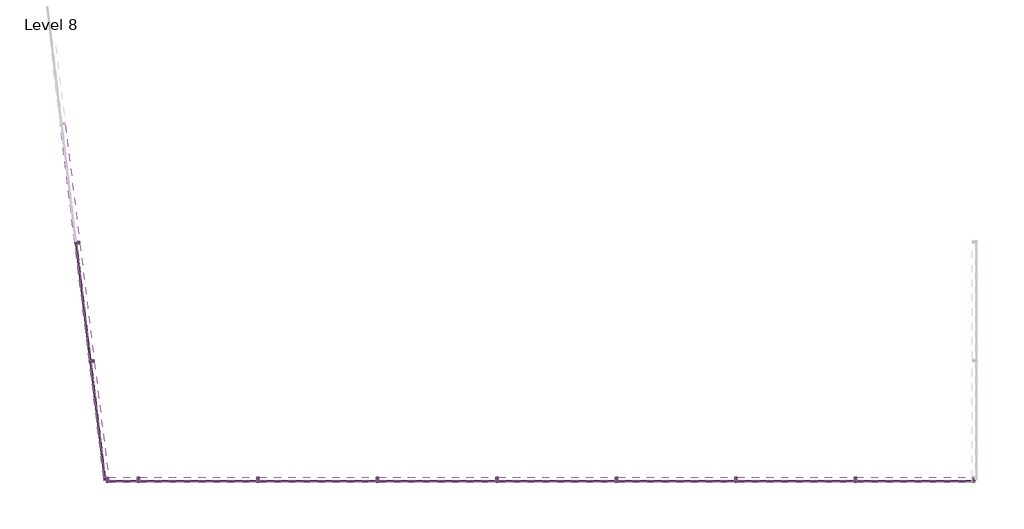
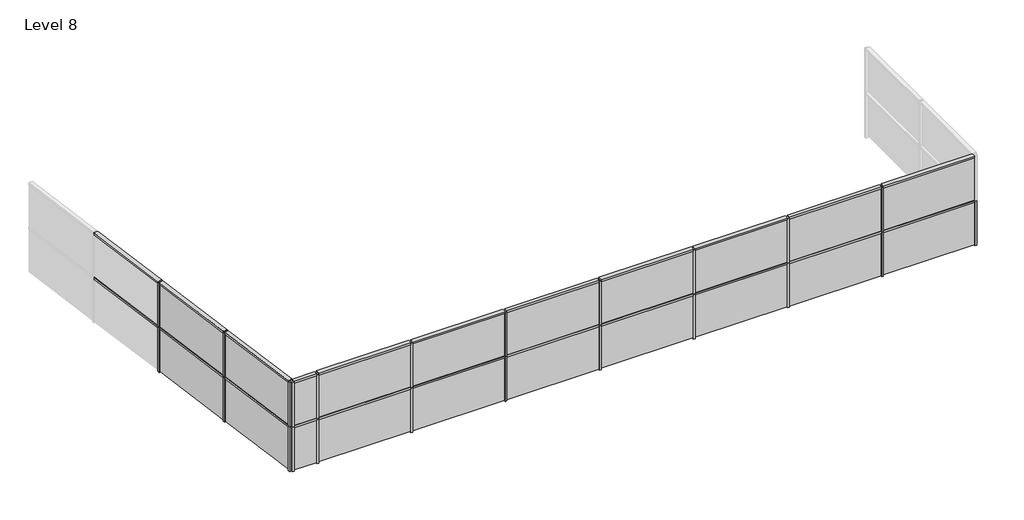
# One storey, part 1 of 2: 45 members, 20 plates.
"""IFC4 building model written with IfcOpenShell, lengths in millimetres."""

from ifc_helpers import new_model, si_unit, origin, place, context, project, spatial, transform, mapped, element, save
from components import member_19d0a4ec, member_8cef0660, member_82905deb, member_4491d118, member_0c11e56c, system_panel_glazed_e46d4b42, system_panel_glazed_2a6c68b7, system_panel_glazed_9d0e0944

model = new_model("IFC4")

# Units and contexts
model_context = context("Model", 3, world=origin())
ifc_project = project(units=[si_unit("LENGTHUNIT", "METRE", prefix="MILLI")], contexts=[model_context])

# Site, building, storey
site = spatial("IfcSite", under=ifc_project)
building = spatial("IfcBuilding", under=site)
storey = spatial("IfcBuildingStorey", under=building, Name="Level 8", Elevation=21336.0)

# Members
placement = place(None, origin())
member_shape = member_19d0a4ec(model_context)
element("IfcMember", 1, ObjectType="Rectangular Mullion : 2.5\" x 5\" rectangular", at=placement, inside=storey, context=model_context, shape_type="MappedRepresentation", body=[
    mapped(member_shape, transform((13839.0156363, -6979.1363705, 22860.0), x_axis=(0.0, 0.0, 1.0), y_axis=(0.0, -1.0, 0.0), z_axis=(1.0, 0.0, 0.0))),
])
element("IfcMember", 2, ObjectType="Rectangular Mullion : 2.5\" x 5\" rectangular", at=placement, inside=storey, context=model_context, shape_type="MappedRepresentation", body=[
    mapped(member_shape, transform((13839.0156363, -6979.1363705, 24384.0), x_axis=(0.0, 0.0, 1.0), y_axis=(0.0, -1.0, 0.0), z_axis=(1.0, 0.0, 0.0))),
])
element("IfcMember", 3, ObjectType="Rectangular Mullion : 2.5\" x 5\" rectangular", at=placement, inside=storey, context=model_context, shape_type="MappedRepresentation", body=[
    mapped(member_shape, transform((-8260.4765148, -6916.1096898, 22860.0), x_axis=(0.0, 0.0, 1.0), y_axis=(-0.9925461516413222, -0.12186934340514594, 0.0), z_axis=(0.12186934340514592, -0.9925461516413221, 0.0))),
])
element("IfcMember", 4, ObjectType="Rectangular Mullion : 2.5\" x 5\" rectangular", at=placement, inside=storey, context=model_context, shape_type="MappedRepresentation", body=[
    mapped(member_shape, transform((-8260.4765148, -6916.1096898, 24384.0), x_axis=(0.0, 0.0, 1.0), y_axis=(-0.9925461516413222, -0.12186934340514585, 0.0), z_axis=(0.12186934340514584, -0.9925461516413221, 0.0))),
])
member_2_shape = member_8cef0660(model_context)
element("IfcMember", 5, ObjectType="Rectangular Mullion : 2.5\" x 5\" rectangular", at=placement, inside=storey, context=model_context, shape_type="MappedRepresentation", body=[
    mapped(member_2_shape, transform((10822.765636, -6979.1363705, 22860.0), x_axis=(0.0, 0.0, 1.0), y_axis=(0.0, -1.0, 0.0), z_axis=(1.0, 0.0, 0.0))),
])
element("IfcMember", 6, ObjectType="Rectangular Mullion : 2.5\" x 5\" rectangular", at=placement, inside=storey, context=model_context, shape_type="MappedRepresentation", body=[
    mapped(member_2_shape, transform((7774.765636, -6979.1363705, 22860.0), x_axis=(0.0, 0.0, 1.0), y_axis=(0.0, -1.0, 0.0), z_axis=(1.0, 0.0, 0.0))),
])
element("IfcMember", 7, ObjectType="Rectangular Mullion : 2.5\" x 5\" rectangular", at=placement, inside=storey, context=model_context, shape_type="MappedRepresentation", body=[
    mapped(member_2_shape, transform((4726.765636, -6979.1363705, 22860.0), x_axis=(0.0, 0.0, 1.0), y_axis=(0.0, -1.0, 0.0), z_axis=(1.0, 0.0, 0.0))),
])
element("IfcMember", 8, ObjectType="Rectangular Mullion : 2.5\" x 5\" rectangular", at=placement, inside=storey, context=model_context, shape_type="MappedRepresentation", body=[
    mapped(member_2_shape, transform((1678.765636, -6979.1363705, 22860.0), x_axis=(0.0, 0.0, 1.0), y_axis=(0.0, -1.0, 0.0), z_axis=(1.0, 0.0, 0.0))),
])
element("IfcMember", 9, ObjectType="Rectangular Mullion : 2.5\" x 5\" rectangular", at=placement, inside=storey, context=model_context, shape_type="MappedRepresentation", body=[
    mapped(member_2_shape, transform((-1369.234364, -6979.1363705, 22860.0), x_axis=(0.0, 0.0, 1.0), y_axis=(0.0, -1.0, 0.0), z_axis=(1.0, 0.0, 0.0))),
])
element("IfcMember", 10, ObjectType="Rectangular Mullion : 2.5\" x 5\" rectangular", at=placement, inside=storey, context=model_context, shape_type="MappedRepresentation", body=[
    mapped(member_2_shape, transform((-4417.234364, -6979.1363705, 22860.0), x_axis=(0.0, 0.0, 1.0), y_axis=(0.0, -1.0, 0.0), z_axis=(1.0, 0.0, 0.0))),
])
element("IfcMember", 11, ObjectType="Rectangular Mullion : 2.5\" x 5\" rectangular", at=placement, inside=storey, context=model_context, shape_type="MappedRepresentation", body=[
    mapped(member_2_shape, transform((10822.765636, -6979.1363705, 24384.0), x_axis=(0.0, 0.0, 1.0), y_axis=(0.0, -1.0, 0.0), z_axis=(1.0, 0.0, 0.0))),
])
element("IfcMember", 12, ObjectType="Rectangular Mullion : 2.5\" x 5\" rectangular", at=placement, inside=storey, context=model_context, shape_type="MappedRepresentation", body=[
    mapped(member_2_shape, transform((7774.765636, -6979.1363705, 24384.0), x_axis=(0.0, 0.0, 1.0), y_axis=(0.0, -1.0, 0.0), z_axis=(1.0, 0.0, 0.0))),
])
element("IfcMember", 13, ObjectType="Rectangular Mullion : 2.5\" x 5\" rectangular", at=placement, inside=storey, context=model_context, shape_type="MappedRepresentation", body=[
    mapped(member_2_shape, transform((4726.765636, -6979.1363705, 24384.0), x_axis=(0.0, 0.0, 1.0), y_axis=(0.0, -1.0, 0.0), z_axis=(1.0, 0.0, 0.0))),
])
element("IfcMember", 14, ObjectType="Rectangular Mullion : 2.5\" x 5\" rectangular", at=placement, inside=storey, context=model_context, shape_type="MappedRepresentation", body=[
    mapped(member_2_shape, transform((1678.765636, -6979.1363705, 24384.0), x_axis=(0.0, 0.0, 1.0), y_axis=(0.0, -1.0, 0.0), z_axis=(1.0, 0.0, 0.0))),
])
element("IfcMember", 15, ObjectType="Rectangular Mullion : 2.5\" x 5\" rectangular", at=placement, inside=storey, context=model_context, shape_type="MappedRepresentation", body=[
    mapped(member_2_shape, transform((-1369.234364, -6979.1363705, 24384.0), x_axis=(0.0, 0.0, 1.0), y_axis=(0.0, -1.0, 0.0), z_axis=(1.0, 0.0, 0.0))),
])
element("IfcMember", 16, ObjectType="Rectangular Mullion : 2.5\" x 5\" rectangular", at=placement, inside=storey, context=model_context, shape_type="MappedRepresentation", body=[
    mapped(member_2_shape, transform((-4417.234364, -6979.1363705, 24384.0), x_axis=(0.0, 0.0, 1.0), y_axis=(0.0, -1.0, 0.0), z_axis=(1.0, 0.0, 0.0))),
])
element("IfcMember", 17, ObjectType="Rectangular Mullion : 2.5\" x 5\" rectangular", at=placement, inside=storey, context=model_context, shape_type="MappedRepresentation", body=[
    mapped(member_2_shape, transform((-8628.0649219, -3922.3423596, 22860.0), x_axis=(0.0, 0.0, 1.0), y_axis=(-0.9925461516413222, -0.12186934340514607, 0.0), z_axis=(0.12186934340514607, -0.9925461516413222, 0.0))),
])
element("IfcMember", 18, ObjectType="Rectangular Mullion : 2.5\" x 5\" rectangular", at=placement, inside=storey, context=model_context, shape_type="MappedRepresentation", body=[
    mapped(member_2_shape, transform((-8999.5226806, -897.0616894, 22860.0), x_axis=(0.0, 0.0, 1.0), y_axis=(-0.9925461516413222, -0.12186934340514592, 0.0), z_axis=(0.12186934340514592, -0.9925461516413222, 0.0))),
])
element("IfcMember", 19, ObjectType="Rectangular Mullion : 2.5\" x 5\" rectangular", at=placement, inside=storey, context=model_context, shape_type="MappedRepresentation", body=[
    mapped(member_2_shape, transform((-8628.0649219, -3922.3423596, 24384.0), x_axis=(0.0, 0.0, 1.0), y_axis=(-0.9925461516413222, -0.1218693434051457, 0.0), z_axis=(0.1218693434051457, -0.9925461516413222, 0.0))),
])
element("IfcMember", 20, ObjectType="Rectangular Mullion : 2.5\" x 5\" rectangular", at=placement, inside=storey, context=model_context, shape_type="MappedRepresentation", body=[
    mapped(member_2_shape, transform((-8999.5226806, -897.0616894, 24384.0), x_axis=(0.0, 0.0, 1.0), y_axis=(-0.9925461516413222, -0.12186934340514595, 0.0), z_axis=(0.12186934340514595, -0.9925461516413222, 0.0))),
])
member_3_shape = member_82905deb(model_context)
element("IfcMember", 21, ObjectType="Rectangular Mullion : 2.5\" x 5\" rectangular", at=placement, inside=storey, context=model_context, shape_type="MappedRepresentation", body=[
    mapped(member_3_shape, transform((10854.515636, -6979.1363705, 22860.0), x_axis=(-1.0, 0.0, 0.0), y_axis=(0.0, -1.0, 0.0), z_axis=(0.0, 0.0, 1.0))),
])
element("IfcMember", 22, ObjectType="Rectangular Mullion : 2.5\" x 5\" rectangular", at=placement, inside=storey, context=model_context, shape_type="MappedRepresentation", body=[
    mapped(member_3_shape, transform((10854.515636, -6979.1363705, 24384.0), x_axis=(-1.0, 0.0, 0.0), y_axis=(0.0, -1.0, 0.0), z_axis=(0.0, 0.0, 1.0))),
])
element("IfcMember", 23, ObjectType="Rectangular Mullion : 2.5\" x 5\" rectangular", at=placement, inside=storey, context=model_context, shape_type="MappedRepresentation", body=[
    mapped(member_3_shape, transform((7806.515636, -6979.1363705, 22860.0), x_axis=(-1.0, 0.0, 0.0), y_axis=(0.0, -1.0, 0.0), z_axis=(0.0, 0.0, 1.0))),
])
element("IfcMember", 24, ObjectType="Rectangular Mullion : 2.5\" x 5\" rectangular", at=placement, inside=storey, context=model_context, shape_type="MappedRepresentation", body=[
    mapped(member_3_shape, transform((7806.515636, -6979.1363705, 24384.0), x_axis=(-1.0, 0.0, 0.0), y_axis=(0.0, -1.0, 0.0), z_axis=(0.0, 0.0, 1.0))),
])
element("IfcMember", 25, ObjectType="Rectangular Mullion : 2.5\" x 5\" rectangular", at=placement, inside=storey, context=model_context, shape_type="MappedRepresentation", body=[
    mapped(member_3_shape, transform((4758.515636, -6979.1363705, 22860.0), x_axis=(-1.0, 0.0, 0.0), y_axis=(0.0, -1.0, 0.0), z_axis=(0.0, 0.0, 1.0))),
])
element("IfcMember", 26, ObjectType="Rectangular Mullion : 2.5\" x 5\" rectangular", at=placement, inside=storey, context=model_context, shape_type="MappedRepresentation", body=[
    mapped(member_3_shape, transform((4758.515636, -6979.1363705, 24384.0), x_axis=(-1.0, 0.0, 0.0), y_axis=(0.0, -1.0, 0.0), z_axis=(0.0, 0.0, 1.0))),
])
element("IfcMember", 27, ObjectType="Rectangular Mullion : 2.5\" x 5\" rectangular", at=placement, inside=storey, context=model_context, shape_type="MappedRepresentation", body=[
    mapped(member_3_shape, transform((1710.515636, -6979.1363705, 22860.0), x_axis=(-1.0, 0.0, 0.0), y_axis=(0.0, -1.0, 0.0), z_axis=(0.0, 0.0, 1.0))),
])
element("IfcMember", 28, ObjectType="Rectangular Mullion : 2.5\" x 5\" rectangular", at=placement, inside=storey, context=model_context, shape_type="MappedRepresentation", body=[
    mapped(member_3_shape, transform((1710.515636, -6979.1363705, 24384.0), x_axis=(-1.0, 0.0, 0.0), y_axis=(0.0, -1.0, 0.0), z_axis=(0.0, 0.0, 1.0))),
])
element("IfcMember", 29, ObjectType="Rectangular Mullion : 2.5\" x 5\" rectangular", at=placement, inside=storey, context=model_context, shape_type="MappedRepresentation", body=[
    mapped(member_3_shape, transform((-1337.484364, -6979.1363705, 22860.0), x_axis=(-1.0, 0.0, 0.0), y_axis=(0.0, -1.0, 0.0), z_axis=(0.0, 0.0, 1.0))),
])
element("IfcMember", 30, ObjectType="Rectangular Mullion : 2.5\" x 5\" rectangular", at=placement, inside=storey, context=model_context, shape_type="MappedRepresentation", body=[
    mapped(member_3_shape, transform((-1337.484364, -6979.1363705, 24384.0), x_axis=(-1.0, 0.0, 0.0), y_axis=(0.0, -1.0, 0.0), z_axis=(0.0, 0.0, 1.0))),
])
element("IfcMember", 31, ObjectType="Rectangular Mullion : 2.5\" x 5\" rectangular", at=placement, inside=storey, context=model_context, shape_type="MappedRepresentation", body=[
    mapped(member_3_shape, transform((-4385.484364, -6979.1363705, 22860.0), x_axis=(-1.0, 0.0, 0.0), y_axis=(0.0, -1.0, 0.0), z_axis=(0.0, 0.0, 1.0))),
])
element("IfcMember", 32, ObjectType="Rectangular Mullion : 2.5\" x 5\" rectangular", at=placement, inside=storey, context=model_context, shape_type="MappedRepresentation", body=[
    mapped(member_3_shape, transform((-4385.484364, -6979.1363705, 24384.0), x_axis=(-1.0, 0.0, 0.0), y_axis=(0.0, -1.0, 0.0), z_axis=(0.0, 0.0, 1.0))),
])
element("IfcMember", 33, ObjectType="Rectangular Mullion : 2.5\" x 5\" rectangular", at=placement, inside=storey, context=model_context, shape_type="MappedRepresentation", body=[
    mapped(member_3_shape, transform((-7433.484364, -6979.1363705, 22860.0), x_axis=(-1.0, 0.0, 0.0), y_axis=(0.0, -1.0, 0.0), z_axis=(0.0, 0.0, 1.0))),
])
element("IfcMember", 34, ObjectType="Rectangular Mullion : 2.5\" x 5\" rectangular", at=placement, inside=storey, context=model_context, shape_type="MappedRepresentation", body=[
    mapped(member_3_shape, transform((-7433.484364, -6979.1363705, 24384.0), x_axis=(-1.0, 0.0, 0.0), y_axis=(0.0, -1.0, 0.0), z_axis=(0.0, 0.0, 1.0))),
])
element("IfcMember", 35, ObjectType="Rectangular Mullion : 2.5\" x 5\" rectangular", at=placement, inside=storey, context=model_context, shape_type="MappedRepresentation", body=[
    mapped(member_3_shape, transform((-8624.1955702, -3953.8557, 22860.0), x_axis=(-0.1218693434051459, 0.9925461516413222, 0.0), y_axis=(-0.9925461516413222, -0.1218693434051459, 0.0), z_axis=(0.0, 0.0, 1.0))),
])
element("IfcMember", 36, ObjectType="Rectangular Mullion : 2.5\" x 5\" rectangular", at=placement, inside=storey, context=model_context, shape_type="MappedRepresentation", body=[
    mapped(member_3_shape, transform((-8624.1955702, -3953.8557, 24384.0), x_axis=(-0.1218693434051459, 0.9925461516413222, 0.0), y_axis=(-0.9925461516413222, -0.1218693434051459, 0.0), z_axis=(0.0, 0.0, 1.0))),
])
element("IfcMember", 37, ObjectType="Rectangular Mullion : 2.5\" x 5\" rectangular", at=placement, inside=storey, context=model_context, shape_type="MappedRepresentation", body=[
    mapped(member_3_shape, transform((-8995.6533289, -928.5750297, 22860.0), x_axis=(-0.1218693434051459, 0.9925461516413222, 0.0), y_axis=(-0.9925461516413222, -0.1218693434051459, 0.0), z_axis=(0.0, 0.0, 1.0))),
])
element("IfcMember", 38, ObjectType="Rectangular Mullion : 2.5\" x 5\" rectangular", at=placement, inside=storey, context=model_context, shape_type="MappedRepresentation", body=[
    mapped(member_3_shape, transform((-8995.6533289, -928.5750297, 24384.0), x_axis=(-0.1218693434051459, 0.9925461516413222, 0.0), y_axis=(-0.9925461516413222, -0.1218693434051459, 0.0), z_axis=(0.0, 0.0, 1.0))),
])
member_4_shape = member_4491d118(model_context)
element("IfcMember", 39, ObjectType="Rectangular Mullion : 2.5\" x 5\" rectangular", at=placement, inside=storey, context=model_context, shape_type="MappedRepresentation", body=[
    mapped(member_4_shape, transform((13902.5156363, -6979.1363705, 21336.0), x_axis=(1.0, 0.0, 0.0), y_axis=(0.0, -1.0, 0.0), z_axis=(0.0, 0.0, -1.0))),
])
element("IfcMember", 40, ObjectType="Rectangular Mullion : 2.5\" x 5\" rectangular", at=placement, inside=storey, context=model_context, shape_type="MappedRepresentation", body=[
    mapped(member_4_shape, transform((-8252.7378115, -6979.1363705, 21336.0), x_axis=(0.1218693434051459, -0.9925461516413222, 0.0), y_axis=(-0.9925461516413222, -0.1218693434051459, 0.0), z_axis=(0.0, 0.0, -1.0))),
])
element("IfcMember", 41, ObjectType="Rectangular Mullion : 2.5\" x 5\" rectangular", at=placement, inside=storey, context=model_context, shape_type="MappedRepresentation", body=[
    mapped(member_4_shape, transform((-8252.7378115, -6979.1363705, 22860.0), x_axis=(0.1218693434051459, -0.9925461516413222, 0.0), y_axis=(-0.9925461516413222, -0.1218693434051459, 0.0), z_axis=(0.0, 0.0, -1.0))),
])
element("IfcMember", 42, ObjectType="Rectangular Mullion : 2.5\" x 5\" rectangular", at=placement, inside=storey, context=model_context, shape_type="MappedRepresentation", body=[
    mapped(member_4_shape, transform((-8252.7378115, -6979.1363705, 22860.0), x_axis=(-1.0, 0.0, 0.0), y_axis=(0.0, -1.0, 0.0), z_axis=(0.0, 0.0, 1.0))),
])
element("IfcMember", 43, ObjectType="Rectangular Mullion : 2.5\" x 5\" rectangular", at=placement, inside=storey, context=model_context, shape_type="MappedRepresentation", body=[
    mapped(member_4_shape, transform((-8252.7378115, -6979.1363705, 24384.0), x_axis=(-1.0, 0.0, 0.0), y_axis=(0.0, -1.0, 0.0), z_axis=(0.0, 0.0, 1.0))),
])
member_5_shape = member_0c11e56c(model_context)
element("IfcMember", 44, ObjectType="Rectangular Mullion : 2.5\" x 5\" rectangular", at=placement, inside=storey, context=model_context, shape_type="MappedRepresentation", body=[
    mapped(member_5_shape, transform((-7465.234364, -6979.1363705, 22860.0), x_axis=(0.0, 0.0, 1.0), y_axis=(0.0, -1.0, 0.0), z_axis=(1.0, 0.0, 0.0))),
])
element("IfcMember", 45, ObjectType="Rectangular Mullion : 2.5\" x 5\" rectangular", at=placement, inside=storey, context=model_context, shape_type="MappedRepresentation", body=[
    mapped(member_5_shape, transform((-7465.234364, -6979.1363705, 24384.0), x_axis=(0.0, 0.0, 1.0), y_axis=(0.0, -1.0, 0.0), z_axis=(1.0, 0.0, 0.0))),
])

# Plates
system_panel_glazed_shape = system_panel_glazed_e46d4b42(model_context)
element("IfcPlate", 46, ObjectType="System Panel : Glazed", at=placement, inside=storey, context=model_context, shape_type="MappedRepresentation", body=[
    mapped(system_panel_glazed_shape, transform((-8440.4013667, -5450.739365, 21367.75), x_axis=(-0.1218693434051459, 0.9925461516413222, 0.0), y_axis=(-0.9925461516413222, -0.1218693434051459, 0.0), z_axis=(0.0, 0.0, 1.0))),
])
element("IfcPlate", 47, ObjectType="System Panel : Glazed", at=placement, inside=storey, context=model_context, shape_type="MappedRepresentation", body=[
    mapped(system_panel_glazed_shape, transform((-8440.4013667, -5450.739365, 22891.75), x_axis=(-0.1218693434051459, 0.9925461516413222, 0.0), y_axis=(-0.9925461516413222, -0.1218693434051459, 0.0), z_axis=(0.0, 0.0, 1.0))),
])
element("IfcPlate", 48, ObjectType="System Panel : Glazed", at=placement, inside=storey, context=model_context, shape_type="MappedRepresentation", body=[
    mapped(system_panel_glazed_shape, transform((12362.6406361, -6979.1363705, 21367.75), x_axis=(-1.0, 0.0, 0.0), y_axis=(0.0, -1.0, 0.0), z_axis=(0.0, 0.0, 1.0))),
])
element("IfcPlate", 49, ObjectType="System Panel : Glazed", at=placement, inside=storey, context=model_context, shape_type="MappedRepresentation", body=[
    mapped(system_panel_glazed_shape, transform((12362.6406361, -6979.1363705, 22891.75), x_axis=(-1.0, 0.0, 0.0), y_axis=(0.0, -1.0, 0.0), z_axis=(0.0, 0.0, 1.0))),
])
system_panel_glazed_2_shape = system_panel_glazed_2a6c68b7(model_context)
element("IfcPlate", 50, ObjectType="System Panel : Glazed", at=placement, inside=storey, context=model_context, shape_type="MappedRepresentation", body=[
    mapped(system_panel_glazed_2_shape, transform((-8809.9244496, -2441.2153649, 21367.75), x_axis=(-0.1218693434051459, 0.9925461516413222, 0.0), y_axis=(-0.9925461516413222, -0.1218693434051459, 0.0), z_axis=(0.0, 0.0, 1.0))),
])
element("IfcPlate", 51, ObjectType="System Panel : Glazed", at=placement, inside=storey, context=model_context, shape_type="MappedRepresentation", body=[
    mapped(system_panel_glazed_2_shape, transform((-8809.9244496, -2441.2153649, 22891.75), x_axis=(-0.1218693434051459, 0.9925461516413222, 0.0), y_axis=(-0.9925461516413222, -0.1218693434051459, 0.0), z_axis=(0.0, 0.0, 1.0))),
])
element("IfcPlate", 52, ObjectType="System Panel : Glazed", at=placement, inside=storey, context=model_context, shape_type="MappedRepresentation", body=[
    mapped(system_panel_glazed_2_shape, transform((9330.515636, -6979.1363705, 21367.75), x_axis=(-1.0, 0.0, 0.0), y_axis=(0.0, -1.0, 0.0), z_axis=(0.0, 0.0, 1.0))),
])
element("IfcPlate", 53, ObjectType="System Panel : Glazed", at=placement, inside=storey, context=model_context, shape_type="MappedRepresentation", body=[
    mapped(system_panel_glazed_2_shape, transform((6282.515636, -6979.1363705, 21367.75), x_axis=(-1.0, 0.0, 0.0), y_axis=(0.0, -1.0, 0.0), z_axis=(0.0, 0.0, 1.0))),
])
element("IfcPlate", 54, ObjectType="System Panel : Glazed", at=placement, inside=storey, context=model_context, shape_type="MappedRepresentation", body=[
    mapped(system_panel_glazed_2_shape, transform((3234.515636, -6979.1363705, 21367.75), x_axis=(-1.0, 0.0, 0.0), y_axis=(0.0, -1.0, 0.0), z_axis=(0.0, 0.0, 1.0))),
])
element("IfcPlate", 55, ObjectType="System Panel : Glazed", at=placement, inside=storey, context=model_context, shape_type="MappedRepresentation", body=[
    mapped(system_panel_glazed_2_shape, transform((186.515636, -6979.1363705, 21367.75), x_axis=(-1.0, 0.0, 0.0), y_axis=(0.0, -1.0, 0.0), z_axis=(0.0, 0.0, 1.0))),
])
element("IfcPlate", 56, ObjectType="System Panel : Glazed", at=placement, inside=storey, context=model_context, shape_type="MappedRepresentation", body=[
    mapped(system_panel_glazed_2_shape, transform((-2861.484364, -6979.1363705, 21367.75), x_axis=(-1.0, 0.0, 0.0), y_axis=(0.0, -1.0, 0.0), z_axis=(0.0, 0.0, 1.0))),
])
element("IfcPlate", 57, ObjectType="System Panel : Glazed", at=placement, inside=storey, context=model_context, shape_type="MappedRepresentation", body=[
    mapped(system_panel_glazed_2_shape, transform((-5909.484364, -6979.1363705, 21367.75), x_axis=(-1.0, 0.0, 0.0), y_axis=(0.0, -1.0, 0.0), z_axis=(0.0, 0.0, 1.0))),
])
element("IfcPlate", 58, ObjectType="System Panel : Glazed", at=placement, inside=storey, context=model_context, shape_type="MappedRepresentation", body=[
    mapped(system_panel_glazed_2_shape, transform((9330.515636, -6979.1363705, 22891.75), x_axis=(-1.0, 0.0, 0.0), y_axis=(0.0, -1.0, 0.0), z_axis=(0.0, 0.0, 1.0))),
])
element("IfcPlate", 59, ObjectType="System Panel : Glazed", at=placement, inside=storey, context=model_context, shape_type="MappedRepresentation", body=[
    mapped(system_panel_glazed_2_shape, transform((6282.515636, -6979.1363705, 22891.75), x_axis=(-1.0, 0.0, 0.0), y_axis=(0.0, -1.0, 0.0), z_axis=(0.0, 0.0, 1.0))),
])
element("IfcPlate", 60, ObjectType="System Panel : Glazed", at=placement, inside=storey, context=model_context, shape_type="MappedRepresentation", body=[
    mapped(system_panel_glazed_2_shape, transform((3234.515636, -6979.1363705, 22891.75), x_axis=(-1.0, 0.0, 0.0), y_axis=(0.0, -1.0, 0.0), z_axis=(0.0, 0.0, 1.0))),
])
element("IfcPlate", 61, ObjectType="System Panel : Glazed", at=placement, inside=storey, context=model_context, shape_type="MappedRepresentation", body=[
    mapped(system_panel_glazed_2_shape, transform((186.515636, -6979.1363705, 22891.75), x_axis=(-1.0, 0.0, 0.0), y_axis=(0.0, -1.0, 0.0), z_axis=(0.0, 0.0, 1.0))),
])
element("IfcPlate", 62, ObjectType="System Panel : Glazed", at=placement, inside=storey, context=model_context, shape_type="MappedRepresentation", body=[
    mapped(system_panel_glazed_2_shape, transform((-2861.484364, -6979.1363705, 22891.75), x_axis=(-1.0, 0.0, 0.0), y_axis=(0.0, -1.0, 0.0), z_axis=(0.0, 0.0, 1.0))),
])
element("IfcPlate", 63, ObjectType="System Panel : Glazed", at=placement, inside=storey, context=model_context, shape_type="MappedRepresentation", body=[
    mapped(system_panel_glazed_2_shape, transform((-5909.484364, -6979.1363705, 22891.75), x_axis=(-1.0, 0.0, 0.0), y_axis=(0.0, -1.0, 0.0), z_axis=(0.0, 0.0, 1.0))),
])
system_panel_glazed_3_shape = system_panel_glazed_9d0e0944(model_context)
element("IfcPlate", 64, ObjectType="System Panel : Glazed", at=placement, inside=storey, context=model_context, shape_type="MappedRepresentation", body=[
    mapped(system_panel_glazed_3_shape, transform((-7827.2360878, -6979.1363705, 21367.75), x_axis=(-1.0, 0.0, 0.0), y_axis=(0.0, -1.0, 0.0), z_axis=(0.0, 0.0, 1.0))),
])
element("IfcPlate", 65, ObjectType="System Panel : Glazed", at=placement, inside=storey, context=model_context, shape_type="MappedRepresentation", body=[
    mapped(system_panel_glazed_3_shape, transform((-7827.2360878, -6979.1363705, 22891.75), x_axis=(-1.0, 0.0, 0.0), y_axis=(0.0, -1.0, 0.0), z_axis=(0.0, 0.0, 1.0))),
])

save(model, "model.ifc")

# Revit data of these elements
# Type "Rectangular Mullion : 2.5\" x 5\" rectangular"
#   built-in parameter 1007304 = 0.416667 (stored number, unit not read)
#   built-in parameter 1007301 = 0.104167 (stored number, unit not read)
#   built-in parameter 1007300 = 0.104167 (stored number, unit not read)
# Type "System Panel : Glazed"
#   Construction Type Id = "GSP4R"
#   Analytic Construction = "1/8 in Pilkington single glazing"
#   Visual Light Transmittance = 0.9
#   Solar Heat Gain Coefficient = 0.86
#   Heat Transfer Coefficient (U) = 1.18115 BTU/(h·ft²·°F)
#   Define Thermal Properties by = 1
# Elements 1, 2, 3, 4, 5, 6, 7, 8, 9, 10, 11, 12, 13, 14, 15, 16, 17, 18, 19, 20, 21, 22, 23, 24, 25, 26, 27, 28, 29, 30, 31, 32, 33, 34, 35, 36, 37, 38, 39, 40, 41, 42, 43, 44, 45 (IfcMember, "Rectangular Mullion : 2.5\" x 5\" rectangular")
#   Phase Created = New Construction
#   Materials on its faces: "Aluminum"
# Elements 46, 47, 48, 49, 50, 51, 52, 53, 54, 55, 56, 57, 58, 59, 60, 61, 62, 63, 64, 65 (IfcPlate, "System Panel : Glazed")
#   Phase Created = New Construction
#   Materials on its faces: "Glass"
# Materials
#   "Aluminum": class "Metal", colour RGB 247 247 247, transparency 0, Description = "Aluminum 6061", Cost = 0
#   "Glass": class "Glass", colour RGB 0 128 192, transparency 0.75, Description = "Soda Lime Glass", Cost = 0
